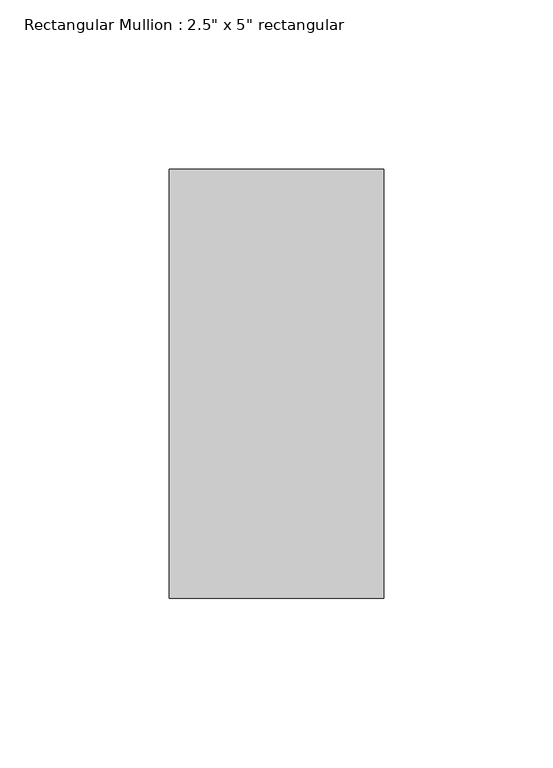
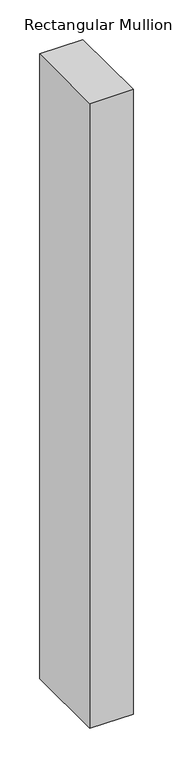
"""IFC4 building model written with IfcOpenShell, lengths in millimetres: member geometry."""

from ifc_helpers import new_model, si_unit, frame, origin, place, context, project, spatial, polyline, outline, extrude, source, transform, mapped, element, save


def member_18e22e2d(model_context):
    return source(origin(), model_context, "Body", "SweptSolid", [
        extrude(outline(polyline([(31.75, 63.5), (31.75, -63.5), (-31.75, -63.5), (-31.75, 63.5), (31.75, 63.5)])), frame((0.0, 0.0, -965.2), z_axis=(0.0, 0.0, 1.0), x_axis=(1.0, 0.0, 0.0)), (0.0, 0.0, 1.0), 965.2),
    ])


if __name__ == "__main__":
    model = new_model("IFC4")
    model_context = context("Model", 3, world=origin())
    ifc_project = project(units=[si_unit("LENGTHUNIT", "METRE", prefix="MILLI")], contexts=[model_context])
    site = spatial("IfcSite", under=ifc_project)
    building = spatial("IfcBuilding", under=site)
    placement = place(None, origin())
    member_shape = member_18e22e2d(model_context)
    element("IfcMember", 1, ObjectType="Rectangular Mullion : 2.5\" x 5\" rectangular", at=placement, inside=building, context=model_context, shape_type="MappedRepresentation", body=[
        mapped(member_shape, transform((0.0, 0.0, 0.0), x_axis=(1.0, 0.0, 0.0), y_axis=(0.0, 1.0, 0.0), z_axis=(0.0, 0.0, 1.0))),
    ])
    save(model, "model.ifc")

# Revit data of these elements
# Type "Rectangular Mullion : 2.5\" x 5\" rectangular"
#   built-in parameter 1007304 = 0.416667 (stored number, unit not read)
#   built-in parameter 1007301 = 0.104167 (stored number, unit not read)
#   built-in parameter 1007300 = 0.104167 (stored number, unit not read)
